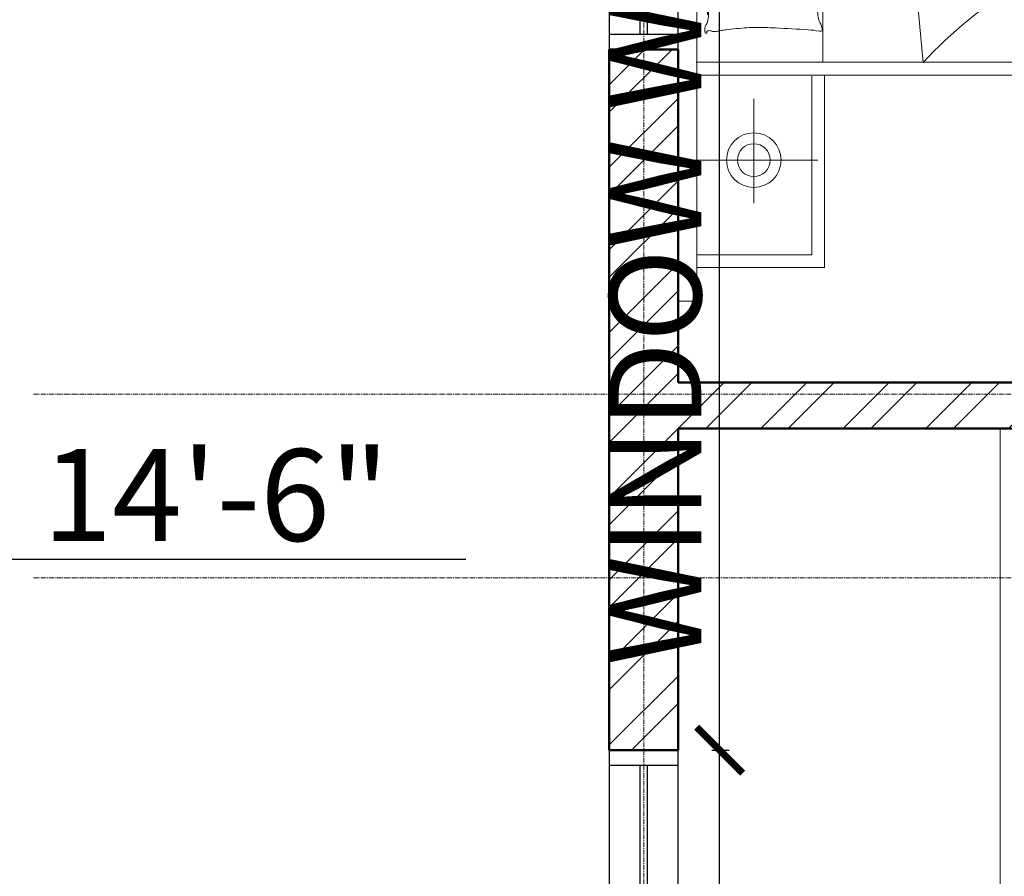
# Model space of a CAD drawing. Units: inches. Extents: x 261 to 2725, y 291 to 1454.
# Tile 20 of 35: x 1166 to 1295, y 741 to 853. Entities that reach past the tile are written whole.
import ezdxf

# ---------------------------------------------------------------- set-up
doc = ezdxf.new("R2010")
doc.units = ezdxf.units.IN
doc.linetypes.add('CENTER', pattern=[2, 1.25, -0.25, 0.25, -0.25])
for name, color, linetype, lineweight in [('A-ANNO-DIMS', 136, 'Continuous', 18), ('A-FLOR-FIXT', 145, 'Continuous', 18), ('A-FURN', 30, 'Continuous', 18), ('A-GLAZ', 150, 'Continuous', 25), ('A-GRID', 251, 'CENTER', 13), ('A-WALL', 222, 'Continuous', 50), ('A-WALL-PATT', 243, 'Continuous', 13)]:
    doc.layers.add(name, color=color, linetype=linetype, lineweight=lineweight)
doc.styles.get("Standard").update_dxf_attribs({"font": 'arial.ttf'})
doc.dimstyles.new('ISO-25', dxfattribs={"dimtxt": 12, "dimasz": 6, "dimexe": 1.25, "dimexo": 0.625, "dimtad": 1, "dimdec": 0, "dimlunit": 3, "dimtxsty": 'Standard', "dimblk": 'ARCHTICK', "dimcen": 2.5, "dimadec": 0, "dimazin": 0, "dimtfac": 1, "dimtdec": 0, "dimtmove": 0, "dimatfit": 3, "dimfxl": 1, "dimfxlon": 1, "dimarcsym": 0})

# ---------------------------------------------------------------- blocks, each defined once
blk = doc.blocks.new('A$C2B723114')
for p, q in [((0, 2.9047), (2.8274, 2.9047)), ((0, 2.8487), (0, 2.9047)), ((2.8274, 2.9047), (2.8274, 2.8487)), ((2.8274, 2.8487), (0, 2.8487)), ((0.1012, 2.4649), (0.1012, 2.849)), ((0.1396, 2.5033), (0.1396, 2.849)), ((0.4243, 2.8697), (0.4243, 2.4855)), ((0.6794, 0.7051), (0.6794, 2.8509)), ((0.7187, 0.7435), (0.7187, 2.8509)), ((2.1776, 2.8509), (2.1776, 0.7454)), ((2.216, 2.8509), (2.216, 0.707)), ((2.4742, 2.8697), (2.4742, 2.4855)), ((2.6798, 2.5052), (2.6798, 2.8509)), ((2.7182, 2.4668), (2.7182, 2.8509)), ((0.6087, 2.6776), (0.295, 2.6776)), ((2.6586, 2.6776), (2.2821, 2.6776)), ((1.3789, 2.4999), (1.3598, 2.5761)), ((2.0593, 2.4999), (2.0402, 2.5761)), ((0.6766, 2.5033), (0.1396, 2.5033)), ((1.3858, 2.4723), (1.3789, 2.4999)), ((2.0662, 2.4723), (2.0593, 2.4999)), ((2.2188, 2.5052), (2.6798, 2.5052)), ((0.6794, 2.4649), (0.1012, 2.4649)), ((0.7191, 2.47), (2.1778, 2.4719)), ((2.2188, 2.4668), (2.7182, 2.4668)), ((2.1771, 2.3036), (0.718, 2.1685)), ((1.0365, 1.6233), (2.1246, 2.2989)), ((2.2287, 1.6076), (2.2523, 1.5035)), ((0.5047, 1.5819), (0.5353, 1.4945)), ((0.6174, 1.5819), (0.6232, 1.4916)), ((0.6467, 1.5819), (0.6369, 1.5137)), ((0.6571, 1.4945), (0.6571, 1.5765)), ((2.2726, 1.593), (2.3061, 1.5007)), ((2.3067, 1.5881), (2.3373, 1.5007)), ((2.4194, 1.5881), (2.4251, 1.4979)), ((2.4487, 1.5881), (2.4389, 1.5199)), ((2.4591, 1.5007), (2.4591, 1.5828)), ((0.4269, 0.0884), (0.4269, 1.4945)), ((0.4269, 1.4945), (0.6794, 1.4945)), ((2.4685, 1.4964), (2.216, 1.5022)), ((2.4685, 1.4964), (2.4685, 0.0903)), ((0.3172, 1.3923), (0.4213, 1.3687)), ((2.4685, 1.4044), (2.5491, 1.3861)), ((2.4596, 1.3659), (2.552, 1.3324)), ((0.3318, 1.3485), (0.4241, 1.3149)), ((0.3367, 1.3143), (0.4241, 1.2838)), ((2.4645, 1.3318), (2.552, 1.3012)), ((2.4645, 1.2928), (2.5548, 1.2871)), ((2.4645, 1.2635), (2.5328, 1.2733)), ((2.4699, 1.2531), (2.552, 1.2163)), ((2.552, 1.2531), (2.4699, 1.2531)), ((2.5435, 1.2276), (2.4699, 1.2163)), ((2.4699, 1.2163), (2.5463, 1.1823)), ((0.3367, 1.2016), (0.427, 1.1959)), ((0.3367, 1.1724), (0.405, 1.1821)), ((0.4241, 1.162), (0.3421, 1.162)), ((0.3421, 1.162), (0.4241, 1.1252)), ((2.5491, 1.1654), (2.467, 1.1597)), ((2.5463, 1.1455), (2.467, 1.1342)), ((2.5491, 1.1342), (2.4699, 1.1201)), ((2.4699, 1.1201), (2.5491, 1.0946)), ((2.5463, 1.1172), (2.4727, 1.0918)), ((2.5491, 1.0946), (2.4699, 1.0635)), ((2.4699, 1.0635), (2.5491, 0.9842)), ((0.4157, 1.0206), (0.3421, 1.0093)), ((0.3421, 1.0093), (0.4185, 0.9754)), ((2.4642, 1.0267), (2.552, 0.9644)), ((2.4699, 0.9785), (2.552, 0.9531)), ((0.4213, 0.9584), (0.3392, 0.9527)), ((2.467, 0.9559), (2.552, 0.9333)), ((0.4185, 0.9386), (0.3392, 0.9272)), ((0.4213, 0.9272), (0.3421, 0.9131)), ((2.4642, 0.9389), (2.4869, 0.9276)), ((2.4869, 0.9276), (2.5265, 0.9163)), ((0.3421, 0.9131), (0.4213, 0.8876)), ((0.4185, 0.9103), (0.3449, 0.8848)), ((2.4642, 0.8908), (2.5152, 0.8483)), ((2.5265, 0.9163), (2.5491, 0.9163)), ((0.4213, 0.8876), (0.3421, 0.8565)), ((0.3421, 0.8565), (0.4213, 0.7772)), ((2.467, 0.8455), (2.5208, 0.8342)), ((2.5152, 0.8483), (2.5491, 0.837)), ((2.5208, 0.8342), (2.552, 0.8285)), ((0.3364, 0.8197), (0.4241, 0.7574)), ((2.4699, 0.8172), (2.4925, 0.7974)), ((2.5491, 0.8087), (2.4699, 0.8172)), ((2.552, 0.8285), (2.5293, 0.8087)), ((0.3421, 0.7716), (0.4241, 0.7461)), ((2.5491, 0.7606), (2.467, 0.7719)), ((2.4925, 0.7974), (2.535, 0.7889)), ((2.535, 0.7889), (2.552, 0.7861)), ((0.3392, 0.7489), (0.4241, 0.7263)), ((2.1776, 0.7454), (0.7187, 0.7435)), ((2.4727, 0.7464), (2.467, 0.7408)), ((2.552, 0.7464), (2.4727, 0.7464)), ((0.359, 0.7206), (0.3987, 0.7093)), ((2.467, 0.7153), (2.5491, 0.7238)), ((0.3987, 0.7093), (0.4213, 0.7093)), ((2.216, 0.707), (0.6794, 0.7051)), ((0.9938, 0.6115), (1.7555, 0.7064)), ((2.5491, 0.6842), (2.4642, 0.6615)), ((2.552, 0.7096), (2.467, 0.6842)), ((0.3421, 0.6601), (0.4213, 0.5808)), ((2.5491, 0.6672), (2.4755, 0.6587)), ((0.3364, 0.6233), (0.4241, 0.561)), ((2.4755, 0.6474), (2.5548, 0.6276)), ((2.4642, 0.6191), (2.4784, 0.6134)), ((2.467, 0.5993), (2.4869, 0.5964)), ((2.4784, 0.6134), (2.5406, 0.6077)), ((2.4869, 0.5964), (2.552, 0.5964)), ((2.5406, 0.6077), (2.552, 0.6134)), ((0.3421, 0.5752), (0.4241, 0.5497)), ((0.3392, 0.5525), (0.4241, 0.5299)), ((2.467, 0.5313), (2.5491, 0.5596)), ((2.467, 0.5087), (2.5548, 0.5342)), ((2.5548, 0.5342), (2.4699, 0.4889)), ((0.359, 0.5242), (0.3987, 0.5129)), ((0.3364, 0.4785), (0.3874, 0.436)), ((1.4523, 0.5021), (1.1305, 0.4537)), ((1.1305, 0.4537), (0.9938, 0.448)), ((0.4213, 0.415), (0.3364, 0.3923)), ((0.3392, 0.4332), (0.393, 0.4219)), ((0.4241, 0.2868), (0.3392, 0.415)), ((0.3874, 0.436), (0.4213, 0.4247)), ((0.393, 0.4219), (0.4241, 0.4162)), ((0.4241, 0.4162), (0.4015, 0.3964)), ((0.3421, 0.4049), (0.3647, 0.3851)), ((0.4213, 0.3964), (0.3421, 0.4049)), ((0.4213, 0.398), (0.3477, 0.3895)), ((0.3647, 0.3851), (0.4072, 0.3766)), ((2.467, 0.4133), (2.552, 0.4019)), ((2.467, 0.2879), (2.552, 0.4076)), ((0.4072, 0.3766), (0.4241, 0.3738)), ((0.4213, 0.3377), (0.3392, 0.3491)), ((0.3392, 0.2925), (0.4213, 0.3009)), ((0.4241, 0.3236), (0.3449, 0.3236)), ((2.4642, 0.3049), (2.5491, 0.2851)), ((2.467, 0.319), (2.5548, 0.3134)), ((0.3477, 0.2571), (0.427, 0.2373)), ((2.4699, 0.2491), (2.501, 0.2491)), ((2.501, 0.2491), (2.5491, 0.2547)), ((0.3506, 0.2231), (0.4128, 0.2175)), ((0.4128, 0.2175), (0.4241, 0.2231)), ((2.467, 0.2179), (2.5605, 0.1981)), ((0.359, 0.2061), (0.4241, 0.2061)), ((2.467, 0.1981), (2.5491, 0.1613)), ((2.467, 0.184), (2.4982, 0.1755)), ((2.4982, 0.1755), (2.5463, 0.1359)), ((0.3392, 0.1042), (0.4213, 0.1325)), ((2.4699, 0.1302), (2.535, 0.1104)), ((0.3392, 0.0815), (0.427, 0.107)), ((0.427, 0.107), (0.3421, 0.0617)), ((2.4685, 0.0903), (0.4269, 0.0884)), ((0.5106, 0.094), (0.5106, 0.0657)), ((0.5417, 0.094), (0.5474, 0.0572)), ((0.713, 0.094), (0.713, 0.0657)), ((0.7334, 0.0943), (0.7503, 0.0434)), ((0.7786, 0.0915), (0.7786, 0.0632)), ((0.956, 0.0943), (0.973, 0.0434)), ((1.0013, 0.0915), (1.0013, 0.0632)), ((1.1338, 0.094), (1.1338, 0.0657)), ((1.1542, 0.0943), (1.1712, 0.0434)), ((1.1995, 0.0915), (1.1995, 0.0632)), ((1.4088, 0.094), (1.4088, 0.0657)), ((1.44, 0.094), (1.4456, 0.0572)), ((1.5674, 0.0962), (1.5844, 0.0453)), ((1.6127, 0.0934), (1.6127, 0.0651)), ((1.7344, 0.0934), (1.7344, 0.0651)), ((1.7655, 0.0934), (1.7712, 0.0566)), ((1.8568, 0.0962), (1.8738, 0.0453)), ((1.9342, 0.0962), (1.9512, 0.0453)), ((1.9795, 0.0934), (1.9795, 0.0651)), ((2.1012, 0.0934), (2.1012, 0.0651)), ((2.1324, 0.0934), (2.138, 0.0566)), ((2.2236, 0.0962), (2.2406, 0.0453)), ((2.2689, 0.0934), (2.2689, 0.0651)), ((2.3906, 0.0934), (2.3906, 0.0651)), ((2.4218, 0.0934), (2.4274, 0.0566)), ((2.4642, 0.0991), (2.5378, 0.0877)), ((2.535, 0.1104), (2.5491, 0.0991)), ((0.5106, 0.0657), (0.5077, 0.0063)), ((0.587, 0.0884), (0.604, 0.0346)), ((0.6512, 0.0884), (0.6682, 0.0346)), ((0.713, 0.0657), (0.7101, 0.0063)), ((0.7786, 0.0632), (0.7843, 0.0066)), ((0.8739, 0.0884), (0.8908, 0.0346)), ((1.0013, 0.0632), (1.007, 0.0066)), ((1.072, 0.0884), (1.089, 0.0346)), ((1.1338, 0.0657), (1.131, 0.0063)), ((1.1995, 0.0632), (1.2052, 0.0066)), ((1.4088, 0.0657), (1.406, 0.0063)), ((1.4853, 0.0884), (1.5023, 0.0346)), ((1.6127, 0.0651), (1.6184, 0.0085)), ((1.6297, 0.0849), (1.624, 0.0028)), ((1.6693, 0.0623), (1.6608, 0.0028)), ((1.6721, 0.0877), (1.6693, 0.0623)), ((1.7344, 0.0651), (1.7316, 0.0057)), ((1.8108, 0.0877), (1.8278, 0.034)), ((1.9795, 0.0651), (1.9852, 0.0085)), ((1.9965, 0.0849), (1.9908, 0.0028)), ((2.0361, 0.0623), (2.0276, 0.0028)), ((2.039, 0.0877), (2.0361, 0.0623)), ((2.1012, 0.0651), (2.0984, 0.0057)), ((2.1777, 0.0877), (2.1946, 0.034)), ((2.2689, 0.0651), (2.2746, 0.0085)), ((2.2859, 0.0849), (2.2802, 0.0028)), ((2.3255, 0.0623), (2.317, 0.0028)), ((2.3284, 0.0877), (2.3255, 0.0623)), ((2.3906, 0.0651), (2.3878, 0.0057)), ((2.467, 0.0877), (2.484, 0.034)), ((2.5378, 0.0877), (2.5463, 0.0821)), ((0.5474, 0.0572), (0.57, 0.0006)), ((0.604, 0.0346), (0.621, 0.0063)), ((0.6682, 0.0346), (0.6851, 0.0063)), ((0.7503, 0.0434), (0.773, 0.0037)), ((0.8908, 0.0346), (0.9078, 0.0063)), ((0.973, 0.0434), (0.9957, 0.0037)), ((1.089, 0.0346), (1.106, 0.0063)), ((1.1712, 0.0434), (1.1939, 0.0037)), ((1.4456, 0.0572), (1.4683, 0.0006)), ((1.5023, 0.0346), (1.5192, 0.0082)), ((1.5844, 0.0453), (1.607, 0.0057)), ((1.7712, 0.0566), (1.7938, 0)), ((1.8278, 0.034), (1.8448, 0.0057)), ((1.8738, 0.0453), (1.8964, 0.0057)), ((1.9512, 0.0453), (1.9739, 0.0057)), ((2.138, 0.0566), (2.1607, 0)), ((2.1946, 0.034), (2.2116, 0.0057)), ((2.2406, 0.0453), (2.2632, 0.0057)), ((2.4274, 0.0566), (2.4501, 0)), ((2.484, 0.034), (2.501, 0.0057))]:
    blk.add_line(p, q)
for centre, radius in [((0.4243, 2.6776), 0.0821), ((2.4742, 2.6776), 0.0821), ((0.4243, 2.6776), 0.0493), ((2.4742, 2.6776), 0.0493)]:
    blk.add_circle(centre, radius)
for centre, radius, start, end in [((0.8078, 2.821), 0.00214, 160.436, 281.8931), ((0.8088, 2.8207), 0.00315, 111.7883, 160.436), ((0.8162, 2.8021), 0.0232, 94.3025, 111.7883), ((0.8091, 2.8151), 0.00394, 21.9904, 101.8931), ((0.7994, 2.8112), 0.0144, 338.579, 21.9904), ((0.8165, 2.7987), 0.0266, 59.3487, 94.3025), ((0.8554, 2.8643), 0.0497, 239.3487, 264.7408), ((0.9202, 3.5684), 0.7568, 264.7408, 268.0921), ((0.8679, 2.7254), 0.0915, 74.0648, 94.2159), ((0.8679, 2.7254), 0.0915, 53.9136, 74.0648), ((0.9466, 3.6164), 0.8051, 270.5757, 274.8018), ((1.0364, 2.548), 0.2671, 87.4614, 94.8018), ((1.042, 2.6745), 0.1405, 79.8101, 87.4614), ((1.1532, 3.2931), 0.488, 259.8101, 263.9133), ((1.2573, 3.0292), 0.2233, 277.5469, 285.744), ((1.3941, 2.5438), 0.281, 98.4372, 105.744), ((1.3747, 2.6748), 0.1486, 90, 98.4372), ((1.3747, 2.74), 0.0833, 78.7276, 90), ((1.3886, 2.8099), 0.0121, 333.4195, 78.7276), ((1.4882, 2.821), 0.00214, 160.436, 281.8931), ((1.4892, 2.8207), 0.00315, 111.7883, 160.436), ((1.4966, 2.8021), 0.0232, 94.3025, 111.7883), ((1.4895, 2.8151), 0.00394, 21.9904, 101.8931), ((1.4798, 2.8112), 0.0144, 338.579, 21.9904), ((1.4969, 2.7987), 0.0266, 59.3487, 94.3025), ((1.5358, 2.8643), 0.0497, 239.3487, 264.7408), ((1.6006, 3.5684), 0.7568, 264.7408, 268.0921), ((1.5483, 2.7254), 0.0915, 74.0648, 94.2159), ((1.5483, 2.7254), 0.0915, 53.9136, 74.0648), ((1.627, 3.6164), 0.8051, 270.5757, 274.8018), ((1.7168, 2.548), 0.2671, 87.4614, 94.8018), ((1.7224, 2.6745), 0.1405, 79.8101, 87.4614), ((1.8336, 3.2931), 0.488, 259.8101, 263.9133), ((1.9377, 3.0292), 0.2233, 277.5469, 285.744), ((2.0745, 2.5438), 0.281, 98.4372, 105.744), ((2.0551, 2.6748), 0.1486, 90, 98.4372), ((2.0551, 2.74), 0.0833, 78.7276, 90), ((2.069, 2.8099), 0.0121, 333.4195, 78.7276), ((0.8409, 2.7949), 0.0302, 158.579, 188.1335), ((1.0356, 2.8227), 0.2268, 188.1335, 192.1095), ((0.9409, 4.189), 1.3777, 268.0921, 270.5757), ((0.8679, 2.7254), 0.0915, 36.1766, 53.9136), ((0.86, 2.6097), 0.2158, 62.7604, 69.1397), ((0.9263, 2.7386), 0.0708, 51.6114, 62.7604), ((0.7461, 2.511), 0.3611, 46.1885, 51.6114), ((1.204, 3.7695), 0.9671, 263.9133, 270), ((1.204, 3.4318), 0.6294, 270, 277.5469), ((1.3713, 2.8186), 0.0315, 274.4002, 333.4195), ((0.923, 2.7382), 0.4535, 0, 6.2324), ((1.5213, 2.7949), 0.0302, 158.579, 188.1335), ((1.716, 2.8227), 0.2268, 188.1335, 192.1095), ((1.6213, 4.189), 1.3777, 268.0921, 270.5757), ((1.5483, 2.7254), 0.0915, 36.1766, 53.9136), ((1.5404, 2.6097), 0.2158, 62.7604, 69.1397), ((1.6067, 2.7386), 0.0708, 51.6114, 62.7604), ((1.4265, 2.511), 0.3611, 46.1885, 51.6114), ((1.8844, 3.7695), 0.9671, 263.9133, 270), ((1.8844, 3.4318), 0.6294, 270, 277.5469), ((2.0517, 2.8186), 0.0315, 274.4002, 333.4195), ((1.6034, 2.7382), 0.4535, 0, 6.2324), ((0.635, 2.7368), 0.1829, 7.6809, 12.1095), ((-0.0181, 2.6487), 0.8418, 3.3687, 7.6809), ((0.8679, 2.7254), 0.0915, 18.4397, 36.1766), ((0.8523, 2.6218), 0.2076, 39.0349, 46.1885), ((1.3154, 2.7368), 0.1829, 7.6809, 12.1095), ((0.6623, 2.6487), 0.8418, 3.3687, 7.6809), ((1.5483, 2.7254), 0.0915, 18.4397, 36.1766), ((1.5327, 2.6218), 0.2076, 39.0349, 46.1885), ((0.9783, 2.7239), 0.0455, 28.3168, 39.0349), ((0.8558, 2.6579), 0.1846, 23.0028, 28.3168), ((1.1884, 2.7382), 0.1881, 350.3156, 0), ((1.6587, 2.7239), 0.0455, 28.3168, 39.0349), ((1.5362, 2.6579), 0.1846, 23.0028, 28.3168), ((1.8688, 2.7382), 0.1881, 350.3156, 0), ((0.1976, 2.6614), 0.6258, 358.3669, 3.3687), ((0.5722, 2.8434), 0.8132, 347.8016, 350.3156), ((0.878, 2.6614), 0.6258, 358.3669, 3.3687), ((1.2526, 2.8434), 0.8132, 347.8016, 350.3156), ((1.6528, 2.6098), 0.2924, 167.8016, 171.9949), ((2.3332, 2.6098), 0.2924, 167.8016, 171.9949), ((-0.4351, 2.6794), 1.2587, 356.945, 358.3669), ((1.9648, 2.5659), 0.6074, 171.9949, 177.3351), ((0.2453, 2.6794), 1.2587, 356.945, 358.3669), ((2.6452, 2.5659), 0.6074, 171.9949, 177.3351), ((-11.7321, 3.2823), 12.5718, 356.49514, 356.94504), ((-11.0517, 3.2823), 12.5718, 356.49514, 356.94504), ((1.4204, 2.5912), 0.0624, 177.3351, 194.0452), ((2.1008, 2.5912), 0.0624, 177.3351, 194.0452), ((1.4917, 3.1364), 0.681, 244.6889, 246.5156), ((2.1721, 3.1364), 0.681, 244.6889, 246.5156), ((0.5206, 2.5319), 0.2961, 350.0016, 356.4951), ((0.9376, 1.4146), 1.0732, 90.2865, 93.574), ((0.9586, -2.7845), 5.2724, 89.0296, 90.2865), ((0.9954, -0.6123), 3.0999, 87.3904, 89.0296), ((1.4917, 3.1364), 0.681, 246.5156, 248.3423), ((1.4917, 3.1364), 0.681, 248.3423, 250.572), ((1.4917, 3.1364), 0.681, 250.572, 252.8018), ((1.201, 2.5319), 0.2961, 350.0016, 356.4951), ((1.618, 1.4146), 1.0732, 90.2865, 93.574), ((1.639, -2.7845), 5.2724, 89.0296, 90.2865), ((1.6758, -0.6123), 3.0999, 87.3904, 89.0296), ((2.1721, 3.1364), 0.681, 246.5156, 248.3423), ((2.1721, 3.1364), 0.681, 248.3423, 250.572), ((2.1721, 3.1364), 0.681, 250.572, 252.8018), ((0.8298, 2.4774), 0.0178, 170.0016, 196.6978), ((0.8139, 2.4726), 0.00122, 196.6978, 277.1204), ((0.8041, 2.5514), 0.0807, 277.1204, 286.2212), ((0.8068, 2.5419), 0.0707, 286.2212, 297.2841), ((0.8584, 2.4419), 0.0418, 102.869, 117.2841), ((0.879, 2.3515), 0.1345, 93.574, 102.869), ((1.0854, 1.364), 1.1216, 85.3824, 87.3904), ((1.28, 3.7729), 1.2952, 265.3824, 267.2509), ((1.228, 2.691), 0.2121, 267.2509, 281.5586), ((1.2975, 2.3514), 0.1345, 83.5659, 101.5586), ((1.3002, 2.3754), 0.1104, 72.6136, 83.5659), ((1.3965, 2.6828), 0.2118, 252.6136, 260.5159), ((1.4027, 2.7202), 0.2496, 260.5159, 265.9171), ((1.385, 2.4721), 0.000845, 265.9171, 14.0449), ((1.5102, 2.4774), 0.0178, 170.0016, 196.6978), ((1.4943, 2.4726), 0.00122, 196.6978, 277.1204), ((1.4845, 2.5514), 0.0807, 277.1204, 286.2212), ((1.4872, 2.5419), 0.0707, 286.2212, 297.2841), ((1.5388, 2.4419), 0.0418, 102.869, 117.2841), ((1.5594, 2.3515), 0.1345, 93.574, 102.869), ((1.7658, 1.364), 1.1216, 85.3824, 87.3904), ((1.9604, 3.7729), 1.2952, 265.3824, 267.2509), ((1.9084, 2.691), 0.2121, 267.2509, 281.5586), ((1.9779, 2.3514), 0.1345, 83.5659, 101.5586), ((1.9806, 2.3754), 0.1104, 72.6136, 83.5659), ((2.0769, 2.6828), 0.2118, 252.6136, 260.5159), ((2.0831, 2.7202), 0.2496, 260.5159, 265.9171), ((2.0654, 2.4721), 0.000845, 265.9171, 14.0449)]:
    blk.add_arc(centre, radius, start, end)
blk.add_ellipse((0.4962, 1.9132), major_axis=(0.4887, -0.4605), ratio=0.503305, start_param=0.491272, end_param=1.591113)
for points, knots in [([(0.6768, 1.3104), (0.6615, 1.3339), (0.6315, 1.3797), (0.604, 1.4501), (0.5417, 1.4748), (0.5064, 1.4871), (0.4848, 1.4945)], [0, 0, 0, 0, 110.980521, 216.571322, 273.316778, 363.252298, 363.252298, 363.252298, 363.252298]), ([(2.5548, 1.4853), (2.5314, 1.4757), (2.5031, 1.4641), (2.4737, 1.4555), (2.4685, 1.454)], [0, 0, 0, 0, 98.452083, 119.481049, 119.481049, 119.481049, 119.481049]), ([(0.427, 1.4678), (0.4036, 1.4582), (0.3693, 1.4441), (0.3335, 1.4344), (0.3221, 1.4313)], [0, 0, 0, 0, 98.452083, 144.639601, 144.639601, 144.639601, 144.639601]), ([(2.552, 1.4598), (2.5309, 1.4545), (2.5031, 1.4475), (2.4753, 1.4406), (2.4685, 1.4389)], [0, 0, 0, 0, 84.638756, 111.94623, 111.94623, 111.94623, 111.94623]), ([(0.4241, 1.4423), (0.4031, 1.437), (0.3691, 1.4284), (0.3351, 1.4199), (0.3221, 1.4167)], [0, 0, 0, 0, 84.638756, 136.955563, 136.955563, 136.955563, 136.955563]), ([(2.2145, 1.4211), (2.233, 1.4246), (2.2636, 1.4303), (2.2761, 1.3837), (2.3429, 1.3967), (2.3949, 1.3342), (2.4474, 1.3031), (2.4698, 1.2898)], [0, 0, 0, 0, 61.886907, 102.717887, 145.699352, 284.082577, 386.765171, 386.765171, 386.765171, 386.765171]), ([(0.6768, 1.286), (0.6567, 1.2911), (0.6145, 1.3017), (0.5543, 1.3533), (0.4816, 1.349), (0.4362, 1.3493), (0.4233, 1.3493)], [0, 0, 0, 0, 80.250278, 168.388677, 295.908361, 346.663112, 346.663112, 346.663112, 346.663112]), ([(0.4233, 1.3445), (0.4367, 1.3385), (0.464, 1.3264), (0.5129, 1.2848), (0.5456, 1.2161), (0.6131, 1.2349), (0.6142, 1.1913), (0.6642, 1.1806), (0.674, 1.144), (0.6817, 1.1154)], [0, 0, 0, 0, 56.745495, 115.23739, 254.956954, 286.678662, 337.828324, 366.201072, 468.500395, 468.500395, 468.500395, 468.500395]), ([(2.2145, 1.319), (2.2295, 1.319), (2.2678, 1.3192), (2.3288, 1.2705), (2.4143, 1.279), (2.4535, 1.2403), (2.4662, 1.2278)], [0, 0, 0, 0, 57.155505, 146.33427, 287.936209, 355.396728, 355.396728, 355.396728, 355.396728]), ([(2.3573, 1.127), (2.3656, 1.1759), (2.3758, 1.2352), (2.3371, 1.1853), (2.3602, 1.1713), (2.3768, 1.1612)], [0, 0, 0, 0, 107.853607, 130.728419, 189.220329, 189.220329, 189.220329, 189.220329]), ([(2.2182, 1.2059), (2.2419, 1.1958), (2.3116, 1.1659), (2.342, 1.0552), (2.4266, 1.0223), (2.4474, 0.9811), (2.462, 0.9684), (2.4698, 0.9616)], [0, 0, 0, 0, 97.73655, 287.59661, 389.176293, 423.403759, 463.679181, 463.679181, 463.679181, 463.679181]), ([(2.2145, 1.1476), (2.2246, 1.1286), (2.2575, 1.0666), (2.3612, 1.0009), (2.431, 0.9336), (2.4662, 0.8996)], [0, 0, 0, 0, 83.02987, 271.460712, 463.033803, 463.033803, 463.033803, 463.033803]), ([(0.6817, 0.8034), (0.6673, 0.8119), (0.6341, 0.8315), (0.5785, 0.8518), (0.5349, 0.8973), (0.4828, 0.9461), (0.4518, 0.9879), (0.4331, 1.013)], [0, 0, 0, 0, 65.318952, 150.437229, 226.833166, 307.58338, 429.454095, 429.454095, 429.454095, 429.454095]), ([(0.4282, 0.9448), (0.4547, 0.9353), (0.496, 0.9206), (0.5223, 0.8436), (0.5628, 0.7946), (0.6113, 0.7575), (0.6214, 0.7173), (0.6539, 0.7022), (0.672, 0.6897), (0.6768, 0.6864)], [0, 0, 0, 0, 102.299436, 159.044876, 303.717955, 348.579152, 391.138254, 454.581655, 477.456496, 477.456496, 477.456496, 477.456496]), ([(2.2145, 0.823), (2.227, 0.8201), (2.261, 0.8121), (2.261, 0.7401), (2.3352, 0.7659), (2.379, 0.6836), (2.4336, 0.6521), (2.4662, 0.6334)], [0, 0, 0, 0, 46.747668, 127.438174, 179.649794, 280.561838, 429.605131, 429.605131, 429.605131, 429.605131]), ([(0.4282, 0.74), (0.4347, 0.7029), (0.444, 0.6496), (0.5194, 0.6274), (0.555, 0.5807), (0.5975, 0.5243), (0.6789, 0.5415), (0.677, 0.5095), (0.6768, 0.5061)], [0, 0, 0, 0, 130.791737, 187.537266, 286.231946, 353.673191, 460.023761, 472.712403, 472.712403, 472.712403, 472.712403]), ([(2.2218, 0.7246), (2.2595, 0.716), (2.3548, 0.6945), (2.4265, 0.6268), (2.4698, 0.586)], [0, 0, 0, 0, 148.665024, 375.555892, 375.555892, 375.555892, 375.555892]), ([(2.3719, 0.6737), (2.3738, 0.6431), (2.3772, 0.5878), (2.3146, 0.6382), (2.3401, 0.7015), (2.2971, 0.6649), (2.2923, 0.6965), (2.289, 0.7176)], [0, 0, 0, 0, 83.446591, 150.887818, 201.642461, 230.015204, 286.760644, 286.760644, 286.760644, 286.760644]), ([(0.6768, 0.6864), (0.7275, 0.655), (0.8251, 0.5944), (0.9391, 0.606), (0.9938, 0.6115)], [0, 0, 0, 0, 225.995823, 434.686543, 434.686543, 434.686543, 434.686543]), ([(2.2145, 0.5167), (2.1764, 0.5522), (2.1051, 0.6184), (1.9357, 0.5803), (1.9385, 0.6342), (1.9388, 0.6395)], [0, 0, 0, 0, 208.073343, 389.01094, 409.01094, 409.01094, 409.01094, 409.01094]), ([(0.6768, 0.5061), (0.7554, 0.4794), (0.8591, 0.4442), (0.9675, 0.4473), (0.9938, 0.448)], [0, 0, 0, 0, 319.374611, 421.61723, 421.61723, 421.61723, 421.61723]), ([(0.4331, 0.4427), (0.4498, 0.4356), (0.4827, 0.4216), (0.5314, 0.3759), (0.632, 0.3884), (0.6996, 0.3513), (0.7423, 0.3278)], [0, 0, 0, 0, 70.931849, 139.556414, 248.154027, 434.709995, 434.709995, 434.709995, 434.709995]), ([(2.4625, 0.1088), (2.4095, 0.1438), (2.2904, 0.2226), (2.0623, 0.1771), (1.9006, 0.2246), (1.7699, 0.2337), (1.6941, 0.2766), (1.5528, 0.2786), (1.4005, 0.2587), (1.2324, 0.3267), (1.059, 0.2939), (0.9218, 0.426), (0.7359, 0.3204), (0.5586, 0.2391), (0.4502, 0.3116), (0.427, 0.3272)], [0, 0, 0, 0, 239.874704, 538.942419, 850.40885, 893.390315, 1047.998294, 1176.505142, 1437.500972, 1637.333004, 1864.324391, 2089.058767, 2248.736533, 2637.953392, 2744.252142, 2744.252142, 2744.252142, 2744.252142]), ([(1.9771, 0.0962), (1.9286, 0.1117), (1.7864, 0.157), (1.5223, 0.1992), (1.2611, 0.141), (1.0527, 0.2023), (0.8859, 0.1885), (0.76, 0.3042), (0.6211, 0.292), (0.5187, 0.3203), (0.4572, 0.3456), (0.4282, 0.3575)], [0, 0, 0, 0, 198.710624, 582.73994, 1031.873213, 1206.082894, 1423.278209, 1655.952104, 1808.744089, 1945.69963, 2068.229211, 2068.229211, 2068.229211, 2068.229211]), ([(0.8474, 0.0943), (0.82, 0.1047), (0.757, 0.1287), (0.6201, 0.1029), (0.4623, 0.1837), (0.4372, 0.2936), (0.4282, 0.3331)], [0, 0, 0, 0, 112.422038, 258.341957, 533.791494, 688.286079, 688.286079, 688.286079, 688.286079]), ([(0.8718, 0.2941), (0.8821, 0.3221), (0.9041, 0.3814), (0.9523, 0.2773), (0.8733, 0.2454), (0.8757, 0.2798), (0.8766, 0.2941)], [0, 0, 0, 0, 82.720021, 175.094899, 237.579423, 282.440623, 282.440623, 282.440623, 282.440623]), ([(1.2715, 0.221), (1.3344, 0.2172), (1.4529, 0.21), (1.2971, 0.2665), (1.2756, 0.2284), (1.2715, 0.221)], [0, 0, 0, 0, 150.888188, 283.977876, 315.699589, 315.699589, 315.699589, 315.699589])]:
    blk.add_open_spline(points, degree=3, knots=knots)
blk = doc.blocks.new('WIN-72')
for p, q in [((955.45, 950.47), (946.45, 950.47)), ((950.45, 950.47), (950.45, 882.47)), ((951.45, 882.47), (951.45, 950.47)), ((946.45, 882.47), (955.45, 882.47))]:
    blk.add_line(p, q)
blk.add_lwpolyline([(955.45, 880.47), (955.45, 952.47), (946.45, 952.47), (946.45, 880.47)], close=True)
blk = doc.blocks.new('WIN-36')
for p, q in [((1252.08, 755.47), (1243.08, 755.47)), ((1247.08, 755.47), (1247.08, 723.47)), ((1248.08, 723.47), (1248.08, 755.47)), ((1243.08, 723.47), (1252.08, 723.47))]:
    blk.add_line(p, q)
blk.add_lwpolyline([(1252.08, 721.47), (1252.08, 757.47), (1243.08, 757.47), (1243.08, 721.47)], close=True)
blk = doc.blocks.new('_ArchTick')
at = {"color": 0, "linetype": 'ByBlock', "const_width": 0.15}
blk.add_lwpolyline([(-0.5, -0.5), (0.5, 0.5)], dxfattribs=at)
blk = doc.blocks.new('*D59')
at = {"layer": 'A-ANNO-DIMS', "color": 0, "lineweight": -2, "ltscale": 0.07, "transparency": 16777216}
for p, q in [((1257.48, 757.47), (1257.48, 946.37)), ((1256.48, 757.47), (1258.73, 757.47)), ((1257.48, 721.47), (1257.48, 757.47)), ((1256.48, 721.47), (1258.73, 721.47))]:
    blk.add_line(p, q, dxfattribs=at)
at = {"layer": 'Defpoints', "color": 0, "ltscale": 0.07, "transparency": 16777216}
for p in [(1252.08, 757.47), (1257.48, 757.47), (1252.08, 721.47)]:
    blk.add_point(p, dxfattribs=at)
at = {"layer": 'A-ANNO-DIMS', "color": 0, "lineweight": -2, "ltscale": 0.07, "transparency": 16777216, "xscale": 6, "yscale": 6, "zscale": 6}
for p, rotation in [((1257.48, 757.47), 90), ((1257.48, 721.47), 270)]:
    blk.add_blockref('_ArchTick', p, dxfattribs=dict(at, rotation=rotation))
at = {"layer": 'A-ANNO-DIMS', "color": 0, "ltscale": 0.07, "transparency": 16777216, "insert": (1250.64, 854.92), "char_height": 12, "attachment_point": 5, "rotation": 90}
blk.add_mtext('WINDOW W3 3\'-0" TYP.', dxfattribs=at)
blk = doc.blocks.new('*D69')
at = {"layer": 'A-ANNO-DIMS', "color": 0, "lineweight": -2, "ltscale": 0.07, "transparency": 16777216}
for p, q in [((772.63, 783.4), (772.63, 781.15)), ((946.45, 783.4), (946.45, 781.15)), ((772.63, 782.4), (946.45, 782.4)), ((946.45, 782.4), (1224.37, 782.4))]:
    blk.add_line(p, q, dxfattribs=at)
at = {"layer": 'Defpoints', "color": 0, "ltscale": 0.07, "transparency": 16777216}
for p in [(772.63, 808.47), (946.45, 808.47), (946.45, 782.4)]:
    blk.add_point(p, dxfattribs=at)
at = {"layer": 'A-ANNO-DIMS', "color": 0, "lineweight": -2, "ltscale": 0.07, "transparency": 16777216, "xscale": 6, "yscale": 6, "zscale": 6, "rotation": 180}
blk.add_blockref('_ArchTick', (772.63, 782.4), dxfattribs=at)
at = {"layer": 'A-ANNO-DIMS', "color": 0, "lineweight": -2, "ltscale": 0.07, "transparency": 16777216, "xscale": 6, "yscale": 6, "zscale": 6}
blk.add_blockref('_ArchTick', (946.45, 782.4), dxfattribs=at)
at = {"layer": 'A-ANNO-DIMS', "color": 0, "ltscale": 0.07, "transparency": 16777216, "insert": (1088.41, 789.23), "char_height": 12, "attachment_point": 5}
blk.add_mtext('DRAWING ROOM SOFA SET 14\'-6"', dxfattribs=at)
blk = doc.blocks.new('*D83')
at = {"layer": 'A-ANNO-DIMS', "color": 0, "lineweight": -2, "ltscale": 0.07, "transparency": 16777216}
for p, q in [((2600.96, 799.47), (2603.21, 799.47)), ((2601.96, 679.47), (2601.96, 799.47)), ((2600.96, 679.47), (2603.21, 679.47))]:
    blk.add_line(p, q, dxfattribs=at)
at = {"layer": 'Defpoints', "color": 0, "ltscale": 0.07, "transparency": 16777216}
for p in [(946.45, 799.47), (2601.96, 799.47), (946.45, 679.47)]:
    blk.add_point(p, dxfattribs=at)
at = {"layer": 'A-ANNO-DIMS', "color": 0, "lineweight": -2, "ltscale": 0.07, "transparency": 16777216, "xscale": 6, "yscale": 6, "zscale": 6}
for p, rotation in [((2601.96, 799.47), 90), ((2601.96, 679.47), 270)]:
    blk.add_blockref('_ArchTick', p, dxfattribs=dict(at, rotation=rotation))
at = {"layer": 'A-ANNO-DIMS', "color": 0, "ltscale": 0.07, "transparency": 16777216, "insert": (2595.21, 739.47), "char_height": 12, "attachment_point": 5, "rotation": 90}
blk.add_mtext('10\'-0"', dxfattribs=at)
blk = doc.blocks.new('*D84')
at = {"layer": 'A-ANNO-DIMS', "color": 0, "lineweight": -2, "ltscale": 0.07, "transparency": 16777216}
for p, q in [((2600.96, 1024.47), (2603.21, 1024.47)), ((2601.96, 799.47), (2601.96, 1024.47)), ((2600.96, 799.47), (2603.21, 799.47))]:
    blk.add_line(p, q, dxfattribs=at)
at = {"layer": 'Defpoints', "color": 0, "ltscale": 0.07, "transparency": 16777216}
for p in [(946.45, 1024.47), (2601.96, 1024.47), (946.45, 799.47)]:
    blk.add_point(p, dxfattribs=at)
at = {"layer": 'A-ANNO-DIMS', "color": 0, "lineweight": -2, "ltscale": 0.07, "transparency": 16777216, "xscale": 6, "yscale": 6, "zscale": 6}
for p, rotation in [((2601.96, 1024.47), 90), ((2601.96, 799.47), 270)]:
    blk.add_blockref('_ArchTick', p, dxfattribs=dict(at, rotation=rotation))
at = {"layer": 'A-ANNO-DIMS', "color": 0, "ltscale": 0.07, "transparency": 16777216, "insert": (2595.21, 911.97), "char_height": 12, "attachment_point": 5, "rotation": 90}
blk.add_mtext('18\'-9"', dxfattribs=at)
blk = doc.blocks.new('*D103')
at = {"layer": 'A-ANNO-DIMS', "color": 0, "lineweight": -2, "ltscale": 0.07, "transparency": 16777216}
for p, q in [((287.06, 1231.47), (284.81, 1231.47)), ((286.06, 439.47), (286.06, 1231.47)), ((287.06, 439.47), (284.81, 439.47))]:
    blk.add_line(p, q, dxfattribs=at)
at = {"layer": 'Defpoints', "color": 0, "ltscale": 0.07, "transparency": 16777216}
for p in [(286.06, 1231.47), (1243.08, 1231.47), (1243.08, 439.47)]:
    blk.add_point(p, dxfattribs=at)
at = {"layer": 'A-ANNO-DIMS', "color": 0, "lineweight": -2, "ltscale": 0.07, "transparency": 16777216, "xscale": 6, "yscale": 6, "zscale": 6}
for p, rotation in [((286.06, 1231.47), 90), ((286.06, 439.47), 270)]:
    blk.add_blockref('_ArchTick', p, dxfattribs=dict(at, rotation=rotation))
at = {"layer": 'A-ANNO-DIMS', "color": 0, "ltscale": 0.07, "transparency": 16777216, "insert": (279.3, 835.47), "char_height": 12, "attachment_point": 5, "rotation": 90}
blk.add_mtext('66\'-0"', dxfattribs=at)
blk = doc.blocks.new('*D108')
at = {"layer": 'A-ANNO-DIMS', "color": 0, "lineweight": -2, "ltscale": 0.07, "transparency": 16777216}
for p, q in [((287.06, 799.47), (284.81, 799.47)), ((286.06, 673.47), (286.06, 799.47)), ((287.06, 673.47), (284.81, 673.47))]:
    blk.add_line(p, q, dxfattribs=at)
at = {"layer": 'Defpoints', "color": 0, "ltscale": 0.07, "transparency": 16777216}
for p in [(286.06, 799.47), (1252.08, 799.47), (1252.08, 673.47)]:
    blk.add_point(p, dxfattribs=at)
at = {"layer": 'A-ANNO-DIMS', "color": 0, "lineweight": -2, "ltscale": 0.07, "transparency": 16777216, "xscale": 6, "yscale": 6, "zscale": 6}
for p, rotation in [((286.06, 799.47), 90), ((286.06, 673.47), 270)]:
    blk.add_blockref('_ArchTick', p, dxfattribs=dict(at, rotation=rotation))
at = {"layer": 'A-ANNO-DIMS', "color": 0, "ltscale": 0.07, "transparency": 16777216, "insert": (279.3, 736.47), "char_height": 12, "attachment_point": 5, "rotation": 90}
blk.add_mtext('10\'-6"', dxfattribs=at)
blk = doc.blocks.new('*D109')
at = {"layer": 'A-ANNO-DIMS', "color": 0, "lineweight": -2, "ltscale": 0.07, "transparency": 16777216}
for p, q in [((287.06, 964.47), (284.81, 964.47)), ((286.06, 799.47), (286.06, 964.47)), ((287.06, 799.47), (284.81, 799.47))]:
    blk.add_line(p, q, dxfattribs=at)
at = {"layer": 'Defpoints', "color": 0, "ltscale": 0.07, "transparency": 16777216}
for p in [(286.06, 964.47), (1252.08, 964.47), (1252.08, 799.47)]:
    blk.add_point(p, dxfattribs=at)
at = {"layer": 'A-ANNO-DIMS', "color": 0, "lineweight": -2, "ltscale": 0.07, "transparency": 16777216, "xscale": 6, "yscale": 6, "zscale": 6}
for p, rotation in [((286.06, 964.47), 90), ((286.06, 799.47), 270)]:
    blk.add_blockref('_ArchTick', p, dxfattribs=dict(at, rotation=rotation))
at = {"layer": 'A-ANNO-DIMS', "color": 0, "ltscale": 0.07, "transparency": 16777216, "insert": (279.3, 881.97), "char_height": 12, "attachment_point": 5, "rotation": 90}
blk.add_mtext('13\'-9"', dxfattribs=at)
blk = doc.blocks.new('*D123')
at = {"layer": 'A-ANNO-DIMS', "color": 0, "lineweight": -2, "ltscale": 0.07, "transparency": 16777216}
for p, q in [((287.06, 1054.85), (284.81, 1054.85)), ((286.06, 439.47), (286.06, 1054.85)), ((287.06, 439.47), (284.81, 439.47))]:
    blk.add_line(p, q, dxfattribs=at)
at = {"layer": 'Defpoints', "color": 0, "ltscale": 0.07, "transparency": 16777216}
for p in [(286.06, 1054.85), (2007.71, 1054.85), (2007.71, 439.47)]:
    blk.add_point(p, dxfattribs=at)
at = {"layer": 'A-ANNO-DIMS', "color": 0, "lineweight": -2, "ltscale": 0.07, "transparency": 16777216, "xscale": 6, "yscale": 6, "zscale": 6}
for p, rotation in [((286.06, 1054.85), 90), ((286.06, 439.47), 270)]:
    blk.add_blockref('_ArchTick', p, dxfattribs=dict(at, rotation=rotation))
at = {"layer": 'A-ANNO-DIMS', "color": 0, "ltscale": 0.07, "transparency": 16777216, "insert": (279.22, 747.16), "char_height": 12, "attachment_point": 5, "rotation": 90}
blk.add_mtext('51\'-3 1/2"', dxfattribs=at)

msp = doc.modelspace()

# ---------------------------------------------------------------- hatches: boundary and pattern name
at = {"layer": 'A-WALL-PATT'}
h = msp.add_hatch(dxfattribs=at)
h.set_pattern_fill('ANSI32', color=256, scale=0.8)
h.paths.add_polyline_path([(478.45, 685.47), (580.45, 685.47), (580.45, 691.47), (577.45, 691.47), (577.45, 694.47), (571.45, 694.47), (571.45, 691.47), (478.45, 691.47), (478.45, 721.47), (469.45, 721.47), (469.45, 508.47), (538.45, 508.47), (538.45, 517.47), (478.45, 517.47)])
h.paths.add_polyline_path([(694.45, 517.47), (676.45, 517.47), (676.45, 646.47), (670.45, 646.47), (670.45, 517.47), (610.45, 517.47), (610.45, 508.47), (694.45, 508.47)])
h.paths.add_polyline_path([(676.45, 784.47), (478.45, 784.47), (478.45, 844.47), (469.45, 844.47), (469.45, 745.47), (478.45, 745.47), (478.45, 775.47), (571.45, 775.47), (571.45, 724.47), (577.45, 724.47), (577.45, 775.47), (670.45, 775.47), (670.45, 691.47), (610.45, 691.47), (610.45, 685.47), (670.45, 685.47), (670.45, 682.47), (676.45, 682.47)])
h.paths.add_polyline_path([(955.45, 880.47), (946.45, 880.47), (946.45, 808.47), (778.45, 808.47), (778.45, 799.47), (946.45, 799.47), (946.45, 517.47), (898.45, 517.47), (898.45, 508.47), (955.45, 508.47)])
h.paths.add_polyline_path([(778.45, 598.47), (772.45, 598.47), (772.45, 517.47), (754.45, 517.47), (754.45, 508.47), (826.45, 508.47), (826.45, 517.47), (778.45, 517.47)])
h.paths.add_polyline_path([(955.45, 1090.47), (946.45, 1090.47), (946.45, 1030.47), (817.45, 1030.47), (817.45, 1024.47), (946.45, 1024.47), (946.45, 952.47), (955.45, 952.47)])
h.paths.add_polyline_path([(955.45, 1231.47), (730.45, 1231.47), (730.45, 1222.47), (772.45, 1222.47), (772.45, 1096.47), (766.45, 1096.47), (766.45, 1090.47), (772.45, 1090.47), (772.45, 1006.47), (712.45, 1006.47), (712.45, 1000.47), (778.45, 1000.47), (778.45, 1024.47), (781.45, 1024.47), (781.45, 1030.47), (778.45, 1030.47), (778.45, 1222.47), (946.45, 1222.47), (946.45, 1162.47), (955.45, 1162.47)])
h.paths.add_polyline_path([(694.45, 1231.47), (619.45, 1231.47), (619.45, 1222.47), (646.45, 1222.47), (646.45, 1039.47), (652.45, 1039.47), (652.45, 1090.47), (736.45, 1090.47), (736.45, 1096.47), (652.45, 1096.47), (652.45, 1222.47), (694.45, 1222.47)])
h.paths.add_polyline_path([(571.45, 1231.47), (469.45, 1231.47), (469.45, 1099.47), (478.45, 1099.47), (478.45, 1144.47), (544.45, 1144.47), (544.45, 1153.47), (538.45, 1153.47), (538.45, 1150.47), (478.45, 1150.47), (478.45, 1222.47), (538.45, 1222.47), (538.45, 1183.47), (544.45, 1183.47), (544.45, 1222.47), (571.45, 1222.47)])
h.paths.add_polyline_path([(538.45, 1006.47), (478.45, 1006.47), (478.45, 1051.47), (469.45, 1051.47), (469.45, 940.47), (478.45, 940.47), (478.45, 1000.47), (538.45, 1000.47)])
h.paths.add_polyline_path([(652.45, 1006.47), (652.45, 1009.47), (646.45, 1009.47), (646.45, 1006.47), (586.45, 1006.47), (586.45, 1000.47), (652.45, 1000.47)])
h.paths.add_polyline_path([(1288.08, 973.47), (1243.08, 973.47), (1243.08, 920.97), (1252.08, 920.97), (1252.08, 964.47), (1288.08, 964.47)], flags=17)
h.paths.add_polyline_path([(1402.08, 805.47), (1252.08, 805.47), (1252.08, 848.97), (1243.08, 848.97), (1243.08, 757.47), (1252.08, 757.47), (1252.08, 799.47), (1294.08, 799.47), (1372.08, 799.47), (1372.08, 779.47), (1372.08, 715.47), (1378.08, 715.47), (1378.08, 799.47), (1402.08, 799.47)])
h.paths.add_polyline_path([(1252.08, 721.47), (1243.08, 721.47), (1243.08, 439.47), (1729.08, 439.47), (1729.08, 709.47), (1720.08, 709.47), (1720.08, 679.47), (1582.08, 679.47), (1582.08, 670.47), (1588.08, 670.47), (1588.08, 673.47), (1720.08, 673.47), (1720.08, 559.47), (1690.08, 559.47), (1690.08, 550.47), (1720.08, 550.47), (1720.08, 448.47), (1252.08, 448.47), (1252.08, 496.47), (1312.08, 496.47), (1312.08, 505.47), (1252.08, 505.47), (1252.08, 673.47), (1405.08, 673.47), (1405.08, 679.47), (1378.08, 679.47), (1378.08, 685.47), (1372.08, 685.47), (1372.08, 679.47), (1252.08, 679.47)])
h.paths.add_polyline_path([(1450.08, 550.47), (1480.08, 550.47), (1480.08, 559.47), (1450.08, 559.47), (1450.08, 679.47), (1441.08, 679.47), (1441.08, 673.47), (1444.08, 673.47), (1444.08, 505.47), (1384.08, 505.47), (1384.08, 496.47), (1450.08, 496.47)], flags=17)
h.paths.add_polyline_path([(1618.08, 559.47), (1588.08, 559.47), (1588.08, 634.47), (1582.08, 634.47), (1582.08, 559.47), (1552.08, 559.47), (1552.08, 550.47), (1618.08, 550.47)], flags=17)
h.paths.add_polyline_path([(1564.08, 964.47), (1630.08, 964.47), (1630.08, 973.47), (1477.08, 973.47), (1477.08, 964.47), (1558.08, 964.47), (1558.08, 926.22), (1558.08, 887.97), (1486.08, 887.97), (1486.08, 881.97), (1558.08, 881.97), (1558.08, 805.47), (1450.08, 805.47), (1450.08, 845.97), (1444.08, 845.97), (1444.08, 805.47), (1438.08, 805.47), (1438.08, 799.47), (1564.08, 799.47)], flags=17)
h.paths.add_polyline_path([(1453.08, 973.47), (1408.08, 973.47), (1408.08, 964.47), (1444.08, 964.47), (1444.08, 881.97), (1450.08, 881.97), (1456.08, 881.97), (1456.08, 887.97), (1450.08, 887.97), (1450.08, 964.47), (1453.08, 964.47)], flags=17)
h.paths.add_polyline_path([(1729.08, 1231.47), (1243.08, 1231.47), (1243.08, 1167.47), (1252.08, 1167.47), (1252.08, 1222.47), (1441.08, 1222.47), (1441.08, 1045.47), (1648.08, 1045.47), (1648.08, 1051.47), (1450.08, 1051.47), (1450.08, 1074.47), (1450.08, 1222.47), (1472.08, 1222.47), (1720.08, 1222.47), (1720.08, 1051.47), (1708.08, 1051.47), (1708.08, 1045.47), (1720.08, 1045.47), (1720.08, 973.47), (1702.08, 973.47), (1702.08, 964.47), (1720.08, 964.47), (1720.08, 769.47), (1729.08, 769.47)])
h.paths.add_polyline_path([(2493.71, 1054.85), (2007.71, 1054.85), (2007.71, 439.47), (2214.67, 439.47), (2214.67, 496.47), (2493.71, 496.47)])
h.paths.add_polyline_path([(2016.71, 1045.85), (2304.71, 1045.85), (2304.71, 841.47), (2310.71, 841.47), (2310.71, 1045.85), (2484.71, 1045.85), (2484.71, 805.47), (2310.71, 805.47), (2310.71, 811.47), (2304.71, 811.47), (2304.71, 799.47), (2484.71, 799.47), (2484.71, 679.47), (2304.71, 679.47), (2304.71, 673.47), (2484.71, 673.47), (2484.71, 505.47), (2208.67, 505.47), (2208.67, 448.47), (2016.71, 448.47), (2016.71, 799.47), (2304.71, 799.47), (2304.71, 805.47), (2016.71, 805.47)], flags=16)

# ---------------------------------------------------------------- linework, layer by layer
at = {"layer": 'A-FLOR-FIXT'}
msp.add_lwpolyline([(1252.08, 679.47), (1294.08, 679.47), (1294.08, 799.47), (1252.08, 799.47)], close=True, dxfattribs=at)
at = {"layer": 'A-GRID', "ltscale": 0.5}
for p, q in [((1247.58, 1330.47), (1247.58, 416.47)), ((1167.93, 803.97), (1791.93, 803.97)), ((1167.93, 779.97), (1791.93, 779.97))]:
    msp.add_line(p, q, dxfattribs=at)
at = {"layer": 'A-WALL'}
for p, q in [((1252.08, 848.97), (1243.08, 848.97)), ((1243.08, 757.47), (1243.08, 848.97)), ((1252.08, 848.97), (1252.08, 805.47)), ((1252.08, 805.47), (1402.08, 805.47)), ((1252.08, 799.47), (1372.08, 799.47)), ((1252.08, 757.47), (1252.08, 799.47)), ((1252.08, 757.47), (1243.08, 757.47))]:
    msp.add_line(p, q, dxfattribs=at)

# ---------------------------------------------------------------- block references
at = {"layer": 'A-FURN', "xscale": 43.4111919502411, "yscale": 43.4111919502411, "zscale": 43.4111919502411, "rotation": 90}
msp.add_blockref('A$C2B723114', (1378.18, 816.1), dxfattribs=at)
at = {"layer": 'A-GLAZ'}
for name, p in [('WIN-72', (296.63, -31.5)), ('WIN-36', (0, 0))]:
    msp.add_blockref(name, p, dxfattribs=at)

# ---------------------------------------------------------------- dimensions: what is measured, and where the dimension line sits
at = {"layer": 'A-ANNO-DIMS', "ltscale": 0.07}
for base, p1, p2, picture, middle in [((286.06, 1231.47), (1243.08, 439.47), (1243.08, 1231.47), '*D103', (279.3, 835.47)), ((286.06, 1054.85), (2007.71, 439.47), (2007.71, 1054.85), '*D123', (279.22, 747.16)), ((2601.96, 1024.47), (946.45, 799.47), (946.45, 1024.47), '*D84', (2595.21, 911.97)), ((286.06, 964.47), (1252.08, 799.47), (1252.08, 964.47), '*D109', (279.3, 881.97)), ((286.06, 799.47), (1252.08, 673.47), (1252.08, 799.47), '*D108', (279.3, 736.47)), ((2601.96, 799.47), (946.45, 679.47), (946.45, 799.47), '*D83', (2595.21, 739.47))]:
    dim = msp.add_linear_dim(base=base, p1=p1, p2=p2, angle=90, dimstyle='ISO-25', override={"dimdec": 1, "dimlfac": 1, "dimrnd": 0, "dimzin": 1, "dimdsep": 46, "dimlunit": 4, "dimfrac": 2}, dxfattribs=at)
    dim.commit()
    dim.dimension.update_dxf_attribs({"geometry": picture, "text_midpoint": middle})
dim = msp.add_linear_dim(base=(1257.48, 757.47), p1=(1252.08, 721.47), p2=(1252.08, 757.47), angle=90, text='WINDOW W3 <> TYP.', dimstyle='ISO-25', override={"dimdec": 1, "dimrnd": 0, "dimzin": 1, "dimlunit": 4, "dimfrac": 2}, dxfattribs=at)
dim.commit()
dim.dimension.update_dxf_attribs({"geometry": '*D59', "text_midpoint": (1250.64, 854.92)})
dim = msp.add_linear_dim(base=(946.45, 782.4), p1=(772.63, 808.47), p2=(946.45, 808.47), text='DRAWING ROOM SOFA SET <>', dimstyle='ISO-25', override={"dimdec": 1, "dimrnd": 0, "dimzin": 1, "dimlunit": 4, "dimfrac": 2}, dxfattribs=at)
dim.commit()
dim.dimension.update_dxf_attribs({"geometry": '*D69', "text_midpoint": (1088.41, 789.23)})

doc.saveas('drawing.dxf')
